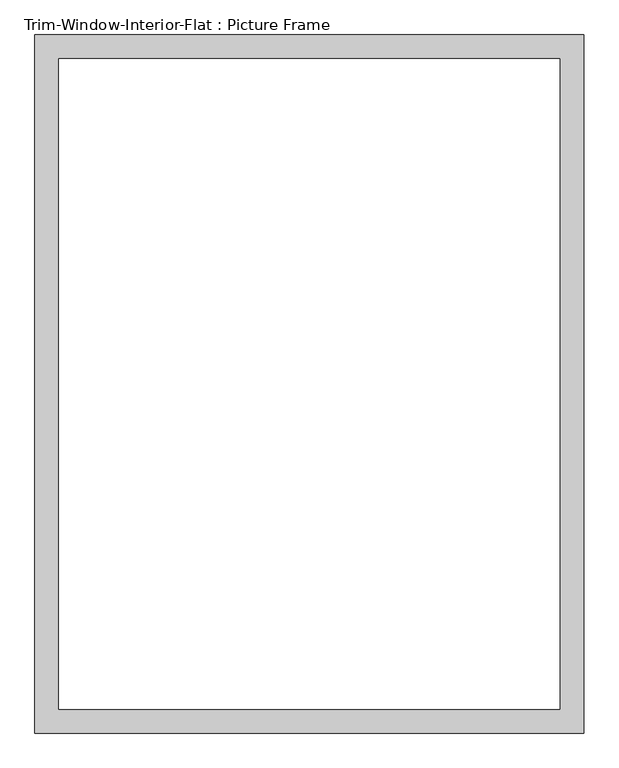
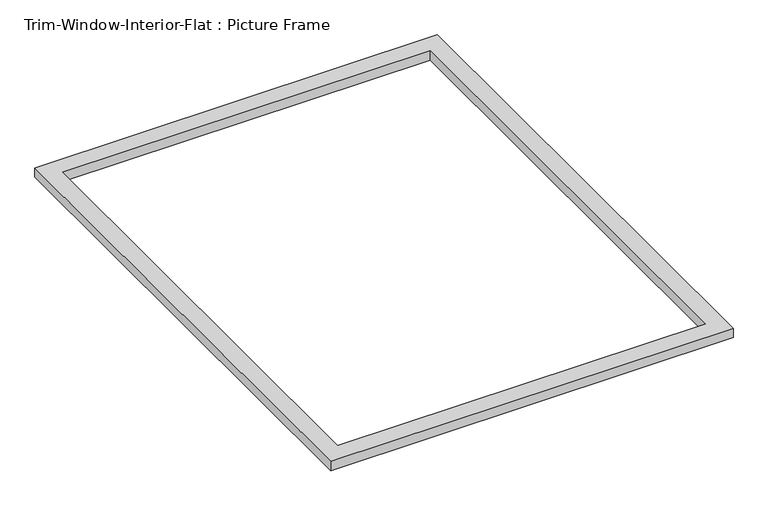
"""IFC4 building model written with IfcOpenShell, lengths in millimetres: proxy geometry, Trim-Window-Interior-Flat : Picture Frame."""

from ifc_helpers import new_model, si_unit, origin, origin_with_axes, place, context, project, spatial, polyline, outline, extrude, source, transform, mapped, element, save


def trim_window_interior_flat_picture_frame_1060724f(model_context):
    return source(origin(), model_context, "Body", "SweptSolid", [
        extrude(outline(polyline([(654.05, 44.45), (654.05, -1619.25), (-654.05, -1619.25), (-654.05, 44.45), (654.05, 44.45)]), holes=[polyline([(596.9, -12.7), (-596.9, -12.7), (-596.9, -1562.1), (596.9, -1562.1), (596.9, -12.7)])]), origin_with_axes(), (0.0, 0.0, 1.0), 31.75),
    ])


if __name__ == "__main__":
    model = new_model("IFC4")
    model_context = context("Model", 3, world=origin())
    ifc_project = project(units=[si_unit("LENGTHUNIT", "METRE", prefix="MILLI")], contexts=[model_context])
    site = spatial("IfcSite", under=ifc_project)
    building = spatial("IfcBuilding", under=site)
    placement = place(None, origin())
    trim_window_interior_flat_picture_frame_shape = trim_window_interior_flat_picture_frame_1060724f(model_context)
    element("IfcBuildingElementProxy", 1, Name="Trim-Window-Interior-Flat : Picture Frame", ObjectType="Trim-Window-Interior-Flat : Picture Frame", at=placement, inside=building, context=model_context, shape_type="MappedRepresentation", body=[
        mapped(trim_window_interior_flat_picture_frame_shape, transform((0.0, 0.0, 0.0), x_axis=(1.0, 0.0, 0.0), y_axis=(0.0, 1.0, 0.0), z_axis=(0.0, 0.0, 1.0))),
    ])
    save(model, "model.ifc")

# Revit data of these elements
# Type "Trim-Window-Interior-Flat : Picture Frame"
#   Trim Thickness_Picture Frame = 0' - 1 1/4"
#   Trim Width = 0' - 2 1/4"
#   Trim Thickness_with Sill = 0' - 0 3/4"
#   Sill Thickness = 0' - 1 1/4"
#   Opening Width [instance default] = 2' - 0"
#   Opening Height [instance default] = 3' - 0"
#   Default Elevation = 4' - 0"
#   Sill = no
#   Picture Frame = yes
#   Trim Material [instance default] = none
# Element 1 (IfcBuildingElementProxy, "Trim-Window-Interior-Flat : Picture Frame")
#   Opening Width = 4' - 0"
#   Opening Height = 5' - 2"
#   Trim Material = Wood - Stained
#   Materials on its faces: "Wood - Stained"
# Materials
#   "Wood - Stained": class "Wood", colour RGB 224 178 126, transparency 0, Cost = 0
